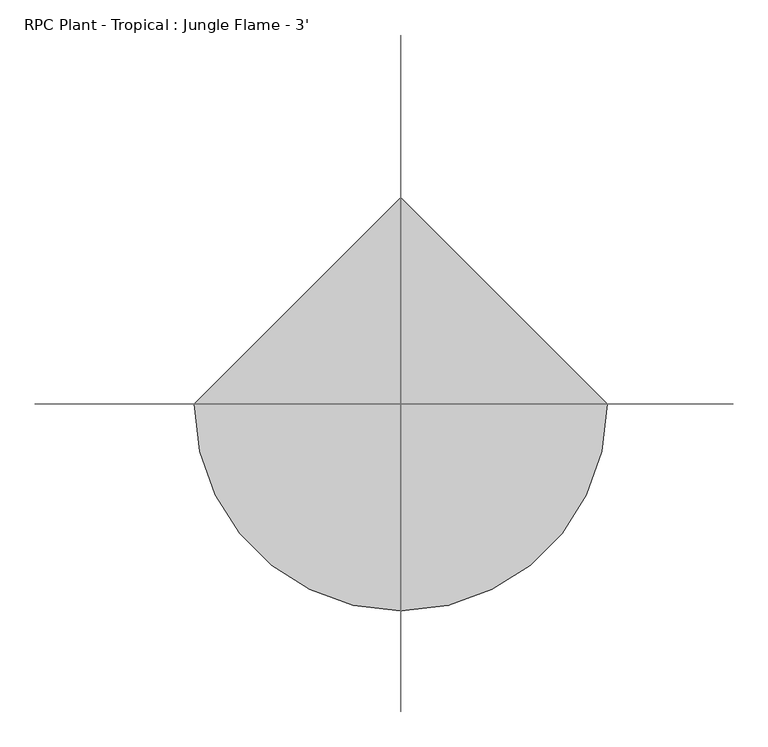
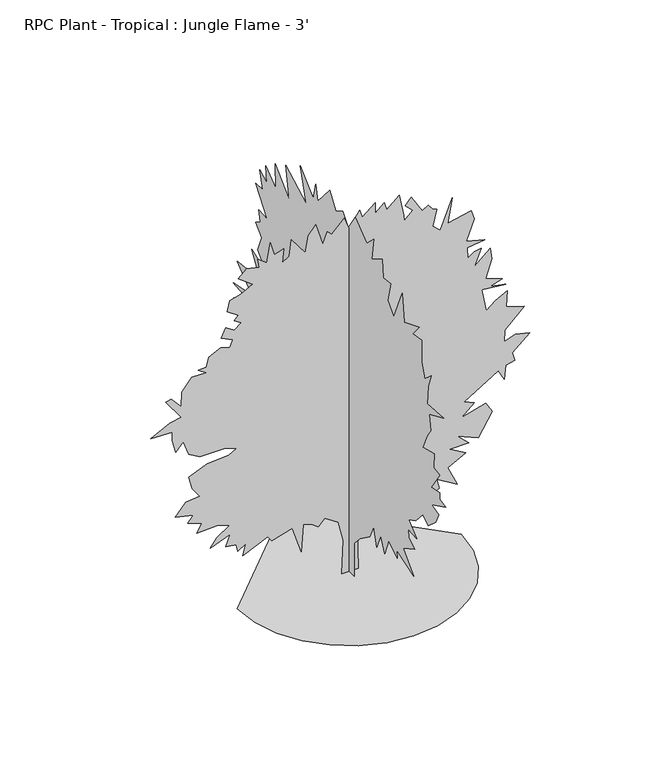
"""IFC4 building model written with IfcOpenShell, lengths in millimetres: geographic element geometry, RPC Plant - Tropical : Jungle Flame - 3'."""

from ifc_helpers import new_model, si_unit, origin, place, context, project, spatial, triangles, source, transform, mapped, element, save


def rpc_plant_tropical_jungle_flame_3_a18473df(model_context):
    return source(origin(), model_context, "Body", "Tessellation", [
        triangles([(-536.1904547, 0.0, 9.29e-05), (-522.0172282, -122.8592432, 9.29e-05), (-481.6464729, -235.6861409, 9.29e-05), (-418.311022, -335.2473784, 9.29e-05), (-335.2473784, -418.3114944, 9.29e-05), (-235.6861409, -481.6464729, 9.29e-05), (-122.8592432, -522.0172282, 9.29e-05), (2.34e-05, -536.1904547, 9.29e-05), (122.8592432, -522.0172282, 9.29e-05), (235.6861409, -481.6464729, 9.29e-05), (335.2473784, -418.311022, 9.29e-05), (418.3114944, -335.2473784, 9.29e-05), (481.6464729, -235.6861409, 9.29e-05), (522.0172282, -122.8592432, 9.29e-05), (536.1904547, 4.69e-05, 9.29e-05), (-7.03e-05, 536.1904547, 9.29e-05), (-2.97e-05, -40.2202966, 8.97e-05), (-2.47e-05, -40.3361053, 168.2066297), (-2.53e-05, -86.8615949, 218.3107116), (-2.71e-05, -169.1754295, 279.1516927), (-2.66e-05, -204.9641244, 350.7286283), (-3.04e-05, -230.0159564, 261.2573453), (-2.95e-05, -262.225691, 339.9922196), (-3.3e-05, -294.4354255, 268.4148118), (-3.19e-05, -326.6451782, 354.3075886), (-3.65e-05, -398.2225679, 307.7824851), (-3.52e-05, -394.6436076, 347.1501403), (-4.28e-05, -534.2198991, 300.6245463), (-3.63e-05, -448.3266681, 390.0962834), (-3.9e-05, -541.3750946, 440.2003836), (-3.59e-05, -491.2751003, 468.8311578), (-3.45e-05, -487.6952316, 508.200666), (-3.78e-05, -559.2698962, 504.6207973), (-3.33e-05, -494.8504272, 561.880529), (-3.5e-05, -552.114737, 590.5149367), (-3.56e-05, -609.3744324, 654.9344421), (-3.84e-05, -655.8991362, 629.8798668), (-3.95e-05, -716.7433147, 683.564308), (-3.91e-05, -741.7933119, 737.244171), (-3.61e-05, -684.5335802, 751.5636457), (-3.95e-05, -799.0575491, 808.8233774), (-3.69e-05, -748.9530493, 819.5584053), (-3.6e-05, -748.9530493, 851.7681398), (-3.34e-05, -680.9537115, 837.4532433), (-3.33e-05, -748.9530493, 941.2421843), (-3.09e-05, -698.8484768, 948.3974161), (-2.89e-05, -702.4283455, 1019.9766226), (-2.54e-05, -609.3744324, 998.5019159), (-2.46e-05, -645.1640356, 1077.2363543), (-2.46e-05, -673.7939014, 1120.1856949), (-2.19e-05, -663.0588736, 1195.3402645), (-2.56e-05, -781.1627838, 1249.024633), (-1.98e-05, -645.1640356, 1238.2896778), (-1.74e-05, -655.8991362, 1334.9188087), (-1.65e-05, -677.3737701, 1399.3382778), (-1.54e-05, -623.6894016, 1352.8091412), (-1.23e-05, -598.6394045, 1420.8084789), (-9e-06, -598.6394045, 1531.7525791), (-6.1e-06, -527.0601617, 1521.0174786), (-6.6e-06, -580.7445665, 1585.4369476), (-2.5e-06, -455.4845887, 1535.3324478), (2.4e-06, -437.5902231, 1671.3311234), (6e-07, -369.5917937, 1510.2825233), (4.5e-06, -319.4876936, 1563.9623863), (6.3e-06, -344.5395075, 1664.171386), (8.8e-06, -283.6989987, 1657.0162994), (1.19e-05, -272.9621178, 1742.9058243), (1.42e-05, -187.069777, 1692.8013245), (1.68e-05, -201.3851641, 1800.1702068), (1.77e-05, -144.1231524, 1746.485693), (2.41e-05, -51.0728955, 1821.6402626), (2.4e-05, 6.1891162, 1732.1707237), (2.78e-05, 52.714247, 1789.4304554), (2.94e-05, 109.9762632, 1757.2207935), (3.38e-05, 160.0803452, 1828.8), (3.48e-05, 260.2885273, 1714.2760311), (3.79e-05, 278.1828747, 1789.4304554), (3.63e-05, 299.6562006, 1703.5409306), (4.41e-05, 407.0218492, 1803.7500755), (3.7e-05, 356.917749, 1642.7013302), (4.73e-05, 525.1261954, 1735.7505924), (4.14e-05, 496.4917514, 1578.2818611), (4.98e-05, 611.0158293, 1689.2259613), (4.6e-05, 607.4405025, 1567.542255), (5.16e-05, 689.7501949, 1631.9617241), (4.88e-05, 682.5950357, 1549.6474171), (5.23e-05, 739.8547674, 1581.8570789), (4.87e-05, 714.8047703, 1495.9675541), (5.13e-05, 775.6443707, 1492.3876854), (4.32e-05, 679.015167, 1367.128616), (4.65e-05, 747.0145048, 1374.2837025), (4.44e-05, 736.2794769, 1320.599334), (4.54e-05, 775.6443707, 1295.5494095), (4.17e-05, 725.5397982, 1245.4447643), (4.08e-05, 757.7495327, 1166.7103987), (3.54e-05, 686.1749044, 1095.1311922), (4.22e-05, 807.8541052, 1138.0805328), (3.42e-05, 721.9599295, 998.5019159), (3.78e-05, 786.3793985, 1023.5564913), (4.35e-05, 925.9580154, 1005.661726), (3.53e-05, 807.8541052, 909.0324497), (4.11e-05, 958.16775, 876.8227152), (3.33e-05, 793.5392086, 862.5078186), (3.13e-05, 775.6443707, 823.138274), (3.88e-05, 954.5878813, 805.2435087), (2.99e-05, 789.9593399, 755.1389362), (2.87e-05, 822.1690744, 665.66947), (2.71e-05, 736.2794769, 740.8240396), (2.39e-05, 711.2249016, 669.2493387), (2.65e-05, 797.1190773, 629.8798668), (2.41e-05, 800.698946, 543.9856911), (1.75e-05, 682.5950357, 497.4610236), (2.01e-05, 768.4892115, 458.0961299), (9.8e-06, 582.3859271, 390.0962834), (1.31e-05, 682.5950357, 350.7286283), (1.33e-05, 739.8547674, 271.9937721), (8.4e-06, 589.5457008, 332.834735), (5.3e-06, 578.8060584, 243.3629797), (4.7e-06, 517.966458, 314.9404058), (-1e-07, 478.601528, 214.7322055), (3.2e-06, 482.1768185, 318.5188937), (2.4e-06, 457.1259493, 329.2557747), (-2.1e-06, 407.0218492, 254.0994246), (-3e-07, 410.6008095, 307.7824851), (-3.9e-06, 324.7080145, 318.5188937), (-4.8e-06, 335.4444231, 271.9937721), (-6.1e-06, 278.1828747, 314.9404058), (-1.09e-05, 260.2885273, 178.9435106), (-1.1e-05, 149.3439184, 343.57118), (-1.27e-05, 124.2916503, 322.097854), (-1.47e-05, 74.1875592, 329.2557747), (-1.53e-05, 102.8187967, 268.4148118), (-1.71e-05, 31.2411618, 314.9404058), (-2.58e-05, 45.5567351, 9.23e-05), (-34.6693841, 0.000106, 3.4e-06), (-27.5516954, 9.57e-05, 167.2634278), (-52.4632448, 9.09e-05, 266.9092532), (-116.5215305, 9.11e-05, 309.6149314), (-148.5506801, 9.45e-05, 277.5857818), (-180.5798206, 9.44e-05, 302.4972336), (-219.7266681, 9.54e-05, 313.1737621), (-230.4027424, 0.0001038, 181.4983329), (-273.1084206, 9.78e-05, 313.1737621), (-369.1958513, 0.0001037, 284.7034614), (-390.5484724, 0.0001029, 313.1737621), (-507.9903591, 0.0001114, 256.2331607), (-493.7531467, 0.0001074, 313.1737621), (-532.8986135, 0.0001106, 288.2623103), (-540.0172196, 0.0001088, 323.8498547), (-589.8428484, 0.0001106, 330.9675525), (-568.4870662, 0.0001062, 387.9081539), (-664.5768042, 0.0001128, 348.7617788), (-632.5453291, 0.0001088, 391.4669847), (-572.048622, 0.0001036, 434.1726628), (-632.5453291, 0.0001052, 451.9664168), (-728.6351034, 0.0001096, 448.4075861), (-703.7222345, 0.0001062, 487.5535252), (-771.3375841, 0.0001077, 512.4663214), (-746.4292934, 0.0001047, 544.4931819), (-831.838833, 0.0001071, 565.8490005), (-782.0177462, 0.0001016, 622.7887299), (-714.397891, 9.82e-05, 629.907336), (-749.9863438, 9.68e-05, 679.7283503), (-767.7805338, 9.37e-05, 743.7866495), (-678.8094383, 8.75e-05, 782.9321526), (-575.6056724, 8.26e-05, 790.0507587), (-536.4602057, 7.96e-05, 811.4065773), (-600.5184686, 8.13e-05, 829.1961891), (-714.397891, 8.63e-05, 829.1961891), (-767.7805338, 8.67e-05, 861.2276642), (-792.69333, 8.36e-05, 932.4045696), (-828.2817827, 8.75e-05, 893.2544884), (-846.0714672, 8.44e-05, 957.3127876), (-846.0714672, 8.19e-05, 1000.0198465), (-949.279775, 8.62e-05, 1003.5768242), (-856.7516293, 7.94e-05, 1049.8455116), (-803.3689865, 7.64e-05, 1060.5210955), (-878.1028696, 7.35e-05, 1163.7248978), (-849.6330231, 7.21e-05, 1167.2818754), (-803.3689865, 7.32e-05, 1113.9038109), (-799.807358, 6.88e-05, 1185.0761381), (-753.5433214, 6.32e-05, 1245.5774597), (-682.3709942, 6.03e-05, 1242.0157585), (-721.5164972, 6.03e-05, 1270.4901833), (-682.3709942, 5.86e-05, 1270.4901833), (-671.6908321, 5.54e-05, 1316.7542198), (-614.7511391, 5.12e-05, 1345.224139), (-572.048622, 5.02e-05, 1330.9869267), (-557.811446, 4.74e-05, 1366.5753067), (-611.1940887, 4.83e-05, 1391.4881756), (-589.8428484, 4.46e-05, 1437.7522121), (-550.6928398, 4.44e-05, 1412.8394886), (-515.1043871, 4.13e-05, 1437.7522121), (-550.6928398, 4.16e-05, 1459.1035252), (-529.3415995, 3.94e-05, 1480.4546928), (-582.7242422, 3.96e-05, 1516.0432182), (-572.048622, 3.6e-05, 1569.425861), (-518.6659793, 3.28e-05, 1583.6630733), (-461.7262862, 2.86e-05, 1612.1329926), (-529.3415995, 2.84e-05, 1665.5156353), (-490.1961328, 2.45e-05, 1701.1040154), (-429.6953198, 2.27e-05, 1686.866803), (-436.8125453, 2.05e-05, 1729.5739346), (-394.1073031, 2.06e-05, 1697.5424595), (-376.3130768, 1.41e-05, 1793.6322338), (-358.5193228, 1.73e-05, 1726.0122334), (-312.2548139, 1.44e-05, 1740.2494457), (-319.3724753, 1.88e-05, 1672.6295906), (-287.3433439, 1.61e-05, 1693.9854092), (-276.6668153, 1.1e-05, 1772.2764153), (-209.0501214, 1.33e-05, 1683.3097527), (-194.8147439, 7.8e-06, 1765.1623146), (-159.2267635, 3.7e-06, 1807.8647953), (-127.1980681, 8.9e-06, 1697.5424595), (-105.8450019, 4.6e-06, 1754.4821526), (-84.4923899, 4.9e-06, 1733.1308395), (-23.9928964, -1.3e-06, 1793.6322338), (-2.6400968, 1.1e-06, 1736.6878899), (50.7418837, -5.5e-06, 1807.8647953), (61.4179626, -3.6e-06, 1768.7193649), (125.4762528, -9.4e-06, 1818.5404518), (125.4762528, -6.2e-06, 1765.1623146), (168.18194, -1.04e-05, 1804.307745), (178.8580144, -8.5e-06, 1765.1623146), (239.3574647, -1.43e-05, 1818.5404518), (260.7105218, -8.7e-06, 1708.218116), (264.2693707, -7.2e-06, 1679.7481968), (303.4157458, -1.12e-05, 1718.898278), (267.8277655, -1.18e-05, 1754.4821526), (296.2985204, -1.49e-05, 1786.5136276), (349.6802911, -1.22e-05, 1701.1040154), (378.1505736, -1.45e-05, 1718.898278), (395.9443276, -1.38e-05, 1693.9854092), (417.2974211, -1.41e-05, 1683.3097527), (399.5031947, -8.6e-06, 1605.0143864), (435.0911751, -8.3e-06, 1572.9874168), (492.0294874, -1.92e-05, 1715.3367222), (470.6782471, -1.11e-05, 1594.3387299), (584.5622114, -1.76e-05, 1619.2514534), (598.7948456, -1.54e-05, 1572.9874168), (559.6493789, -7.8e-06, 1473.3407375), (648.6205107, -1.02e-05, 1448.4278687), (563.2063929, -5.8e-06, 1437.7522121), (566.7679851, -2.8e-06, 1384.3695694), (598.7948456, -5.5e-06, 1405.7208824), (630.826248, -7.3e-06, 1412.8394886), (598.7948456, -1e-06, 1330.9869267), (673.5287287, -8.3e-06, 1398.6067818), (680.6473349, -5.2e-06, 1341.6625832), (652.1774883, 1.3e-06, 1252.6960659), (730.473, -4e-07, 1224.2261467), (673.5287287, 3.2e-06, 1206.4319567), (748.2626844, 1e-06, 1188.637694), (634.3832983, 5.1e-06, 1202.8703281), (655.7345387, 1.09e-05, 1088.990942), (698.4415976, 7e-06, 1124.5793947), (755.3812906, 2.8e-06, 1153.0492413), (751.8242403, 7.6e-06, 1074.7537296), (837.2337799, 5.6e-06, 1046.2838831), (744.7056341, 1.49e-05, 957.3127876), (741.1486565, 1.84e-05, 900.3730946), (794.526721, 1.48e-05, 921.7289131), (862.1465761, 1.29e-05, 903.9347231), (780.2940868, 2.08e-05, 832.7578176), (790.9697433, 2.28e-05, 790.0507587), (748.2626844, 2.53e-05, 779.3751022), (741.1486565, 2.97e-05, 711.7598253), (712.6788099, 2.78e-05, 765.1378899), (548.9737587, 4.08e-05, 665.4957161), (598.7948456, 3.99e-05, 644.1399702), (534.7365463, 4.59e-05, 590.7572548), (652.1774883, 3.89e-05, 622.7887299), (684.2043852, 4.07e-05, 569.4060144), (616.5890356, 5.02e-05, 459.0836786), (516.94232, 5.2e-05, 501.7907012), (570.324999, 5.26e-05, 451.9664168), (481.3538672, 5.67e-05, 448.4075861), (556.0877867, 5.6e-05, 405.7023803), (470.6782471, 6.25e-05, 359.437835), (516.94232, 6.64e-05, 259.7915554), (417.2969487, 6.72e-05, 320.2909876), (431.5323443, 6.95e-05, 270.468084), (360.3563473, 7.45e-05, 238.4389525), (292.7396715, 7.39e-05, 298.9383847), (303.4157458, 8.21e-05, 153.0280322), (264.2693707, 7.6e-05, 284.7034614), (164.6230911, 8.52e-05, 202.850954), (182.4168633, 7.94e-05, 288.2623103), (107.6824897, 8.86e-05, 188.6160307), (86.3294144, 8.57e-05, 252.6743299), (132.5939415, 7.67e-05, 370.1143636), (68.5356513, 8.01e-05, 359.437835), (36.5064608, 8.47e-05, 306.0560643), (43.6240133, 0.0001026, 0.0)], [[15, 16, 1], [14, 15, 1], [14, 1, 2], [13, 14, 2], [13, 2, 3], [13, 3, 4], [12, 13, 4], [11, 12, 4], [11, 4, 5], [11, 5, 6], [11, 6, 7], [11, 7, 8], [11, 8, 9], [11, 9, 10], [101, 102, 103], [119, 120, 121], [51, 52, 53], [104, 105, 106], [76, 77, 78], [27, 28, 29], [59, 60, 61], [106, 107, 108], [78, 79, 80], [122, 123, 124], [61, 62, 63], [54, 55, 56], [131, 132, 133], [115, 116, 117], [114, 115, 117], [21, 22, 23], [40, 41, 42], [32, 33, 34], [96, 97, 98], [68, 69, 70], [125, 126, 127], [127, 128, 129], [82, 83, 84], [86, 87, 88], [112, 113, 114], [23, 24, 25], [99, 100, 101], [84, 85, 86], [117, 118, 119], [80, 81, 82], [25, 26, 27], [88, 89, 90], [29, 30, 31], [44, 45, 46], [66, 67, 68], [64, 65, 66], [90, 91, 92], [46, 47, 48], [74, 75, 76], [92, 93, 94], [42, 43, 44], [40, 42, 44], [38, 39, 40], [98, 99, 101], [57, 58, 59], [70, 71, 72], [133, 134, 17], [133, 17, 18], [133, 18, 19], [104, 106, 108], [114, 117, 119], [72, 73, 74], [133, 19, 20], [37, 38, 40], [36, 37, 40], [133, 20, 21], [110, 111, 112], [109, 110, 112], [44, 46, 48], [53, 54, 56], [94, 95, 96], [98, 101, 103], [90, 92, 94], [68, 70, 72], [114, 119, 121], [114, 121, 122], [98, 103, 104], [129, 130, 131], [64, 66, 68], [86, 88, 90], [84, 86, 90], [82, 84, 90], [25, 27, 29], [25, 29, 31], [25, 31, 32], [57, 59, 61], [57, 61, 63], [56, 57, 63], [53, 56, 63], [98, 104, 108], [49, 50, 51], [36, 40, 44], [36, 44, 48], [35, 36, 48], [34, 35, 48], [25, 32, 34], [23, 25, 34], [21, 23, 34], [21, 34, 48], [133, 21, 48], [131, 133, 48], [129, 131, 48], [90, 94, 96], [82, 90, 96], [80, 82, 96], [109, 112, 114], [109, 114, 122], [64, 68, 72], [122, 124, 125], [109, 122, 125], [109, 125, 127], [109, 127, 129], [109, 129, 48], [108, 109, 48], [98, 108, 48], [96, 98, 48], [80, 96, 48], [78, 80, 48], [76, 78, 48], [74, 76, 48], [72, 74, 48], [64, 72, 48], [63, 64, 48], [53, 63, 48], [53, 48, 49], [53, 49, 51], [252, 253, 254], [236, 237, 238], [284, 285, 286], [141, 142, 143], [241, 242, 243], [204, 205, 206], [174, 175, 176], [151, 152, 153], [279, 280, 281], [266, 267, 268], [183, 184, 185], [250, 251, 252], [151, 153, 154], [286, 287, 288], [202, 203, 204], [209, 210, 211], [275, 276, 277], [145, 146, 147], [218, 219, 220], [220, 221, 222], [247, 248, 249], [288, 289, 290], [288, 290, 291], [155, 156, 157], [262, 263, 264], [212, 213, 214], [211, 212, 214], [245, 246, 247], [244, 245, 247], [171, 172, 173], [277, 278, 279], [261, 262, 264], [224, 225, 226], [256, 257, 258], [177, 178, 179], [177, 179, 180], [258, 259, 260], [222, 223, 224], [159, 160, 161], [269, 270, 271], [247, 249, 250], [216, 217, 218], [214, 215, 216], [206, 207, 208], [147, 148, 149], [250, 252, 254], [159, 161, 162], [157, 158, 159], [229, 230, 231], [228, 229, 231], [193, 194, 195], [149, 150, 151], [199, 200, 201], [199, 201, 202], [190, 191, 192], [189, 190, 192], [294, 135, 136], [293, 294, 136], [293, 136, 137], [204, 206, 208], [174, 176, 177], [264, 265, 266], [231, 232, 233], [238, 239, 240], [238, 240, 241], [236, 238, 241], [138, 139, 140], [255, 256, 258], [255, 258, 260], [163, 164, 165], [281, 282, 283], [281, 283, 284], [273, 274, 275], [272, 273, 275], [271, 272, 275], [233, 234, 235], [231, 233, 235], [162, 163, 165], [162, 165, 166], [143, 144, 145], [195, 196, 197], [195, 197, 198], [227, 228, 231], [227, 231, 235], [171, 173, 174], [171, 174, 177], [261, 264, 266], [261, 266, 268], [195, 198, 199], [293, 137, 138], [292, 293, 138], [157, 159, 162], [155, 157, 162], [155, 162, 166], [154, 155, 166], [154, 166, 167], [286, 288, 291], [284, 286, 291], [181, 182, 183], [180, 181, 183], [247, 250, 254], [147, 149, 151], [185, 186, 187], [185, 187, 188], [183, 185, 188], [199, 202, 204], [199, 204, 208], [224, 226, 227], [277, 279, 281], [277, 281, 284], [277, 284, 291], [261, 268, 269], [189, 192, 193], [236, 241, 243], [193, 195, 199], [193, 199, 208], [145, 147, 151], [145, 151, 154], [145, 154, 167], [143, 145, 167], [141, 143, 167], [222, 224, 227], [275, 277, 291], [271, 275, 291], [269, 271, 291], [177, 180, 183], [140, 141, 167], [138, 140, 167], [292, 138, 167], [291, 292, 167], [269, 291, 167], [261, 269, 167], [260, 261, 167], [255, 260, 167], [254, 255, 167], [247, 254, 167], [244, 247, 167], [243, 244, 167], [236, 243, 167], [235, 236, 167], [227, 235, 167], [222, 227, 167], [220, 222, 167], [218, 220, 167], [216, 218, 167], [214, 216, 167], [211, 214, 167], [209, 211, 167], [208, 209, 167], [193, 208, 167], [189, 193, 167], [188, 189, 167], [183, 188, 167], [177, 183, 167], [177, 167, 168], [171, 177, 168], [171, 168, 169], [170, 171, 169]], closed=False),
    ])


if __name__ == "__main__":
    model = new_model("IFC4")
    model_context = context("Model", 3, world=origin())
    ifc_project = project(units=[si_unit("LENGTHUNIT", "METRE", prefix="MILLI")], contexts=[model_context])
    site = spatial("IfcSite", under=ifc_project)
    building = spatial("IfcBuilding", under=site)
    placement = place(None, origin())
    rpc_plant_tropical_jungle_flame_3_shape = rpc_plant_tropical_jungle_flame_3_a18473df(model_context)
    element("IfcGeographicElement", 1, ObjectType="RPC Plant - Tropical : Jungle Flame - 3'", at=placement, inside=building, context=model_context, shape_type="MappedRepresentation", body=[
        mapped(rpc_plant_tropical_jungle_flame_3_shape, transform((0.0, 0.0, 0.0), x_axis=(1.0, 0.0, 0.0), y_axis=(0.0, 1.0, 0.0), z_axis=(0.0, 0.0, 1.0))),
    ])
    save(model, "model.ifc")

# Revit data of these elements
# Type "RPC Plant - Tropical : Jungle Flame - 3'"
#   built-in parameter 1005198 = "{2, 15},{39, RPC-16-FUVJ-JWG0-MWGK-8000-ST1L-LVER-AU},{1, 0},{1, 0},{2, 35},{1, 8},{5, Color},{1, 0},{1, 0},{3, 0.8},{3, 0.8},{3, 0.8},{1, 8},{7, BBoxMin},{1, 0},{1, 0},{1, 0},{1, 0},{1, 0},{1, 8},{7, BBoxMax},{1, 0},{1, 0},{1, 0},{1, 0},{1, 0},{2, 11},{9, RPCTypeId},{1, 0},{1, 0},{39, RPC-16-FUVJ-JWG0-MWGK-8000-ST1L-LVER-AU},{1, 6},{14, RPCPlantHeight},{1, 0},{1, 0},{1, 3},{2, 11},{7, keyword},{1, 0},{1, 0},{90, :Geometry:RPC:Jungle Flame:ixora macrothyrsa:jungle flame:bush:shrub:plant:flower:tropical},{2, 11},{8, category},{1, 0},{1, 0},{17, :Shrubs [General]},{2, 11},{12, LocalizedUID},{1, 0},{1, 0},{12, Jungle Flame},{2, 14},{6, Height},{1, 0},{1, 0},{1, 3},{1, 2},{16, Cast Reflections},{1, 0},{1, 0},{1, 0},{1, 2},{12, Cast Shadows},{1, 0},{1, 0},{1, 1},{1, 2},{9, Lock View},{1, 0},{1, 0},{1, 0},{1, 4},{5, ViewC},{1, 0},{1, 0},{1, 0},{2, 11},{20, AdvancedUIDefinition},{1, 0},{1, 0},{0, },{2, 11},{10, AssetLibID},{1, 0},{1, 0},{36, 4D3F6E72-3F99-4203-98E9-AF80B3C7A7A4},{2, 11},{10, BaseSchema},{1, 0},{1, 0},{9, RPCSchema},{2, 11},{12, ExchangeGUID},{1, 0},{1, 0},{0, },{1, 2},{6, Hidden},{1, 0},{1, 0},{1, 0},{1, 4},{11, RPCCategory},{1, 0},{1, 0},{1, 0},{2, 11},{8, RPCImage},{1, 0},{1, 0},{0, },{1, 4},{13, SchemaVersion},{1, 0},{1, 0},{1, 4},{2, 11},{12, UIDefinition},{1, 0},{1, 0},{0, },{2, 11},{6, UIName},{1, 0},{1, 0},{39, RPC-16-FUVJ-JWG0-MWGK-8000-ST1L-LVER-AU},{2, 11},{11, VersionGUID},{1, 0},{1, 0},{9, RPCSchema},{2, 11},{9, assettype},{1, 0},{1, 0},{11, RPCGeometry},{2, 11},{11, description},{1, 0},{1, 0},{0, },{2, 11},{9, localname},{1, 0},{1, 0},{3, RPC},{2, 11},{9, localtype},{1, 0},{1, 0},{3, RPC},{1, 4},{8, revision},{1, 0},{1, 0},{1, 1},{2, 11},{9, thumbnail},{1, 0},{1, 0},{0, },{1, 4},{7, version},{1, 0},{1, 0},{1, 1},{1, 2},{20, RPC_Cast Reflections},{1, 0},{1, 0},{1, 1},{1, 2},{16, RPC_Cast Shadows},{1, 0},{1, 0},{1, 1},{1, 2},{13, RPC_Lock View},{1, 0},{1, 0},{1, 0},{1, 4},{9, RPC_ViewC},{1, 0},{1, 0},{1, 0},{21, assetlibrary_base.fbx},{1, 5},"
#   built-in parameter 1005195 = "RPC-16-FUVJ-JWG0-MWGK-8000-ST1L-LVER-AU"
#   Type Comments = "Jungle Flame"
#   Assembly Code = "G2050500"
#   Height = 6' - 0"
#   Default Elevation = 0
